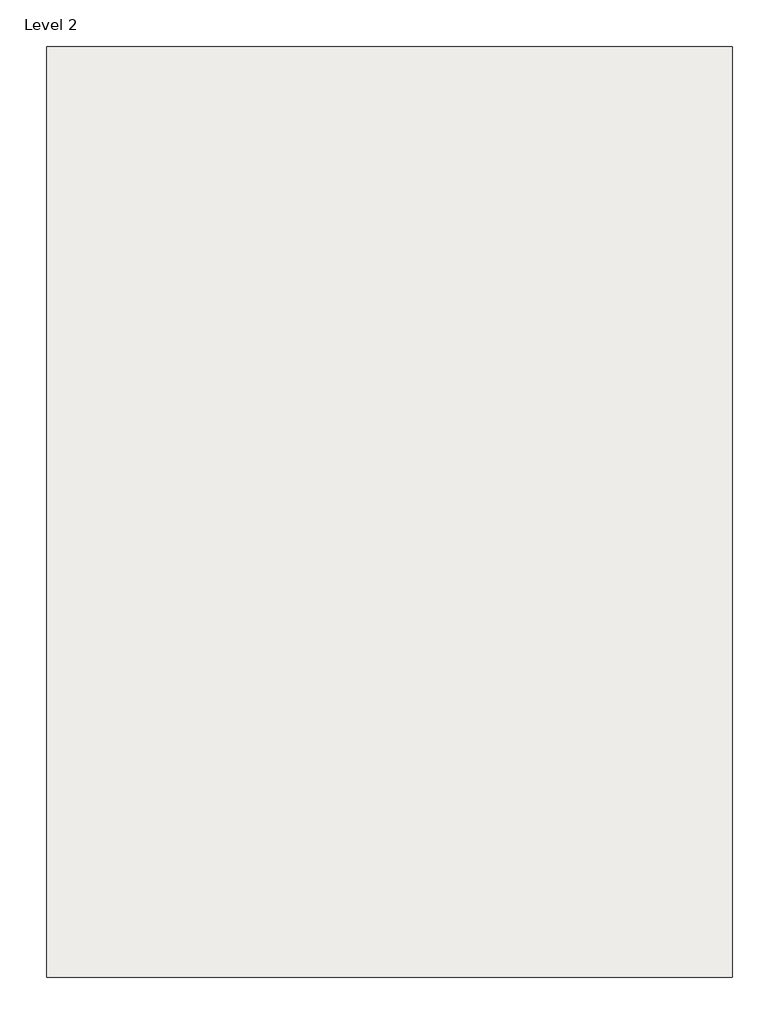
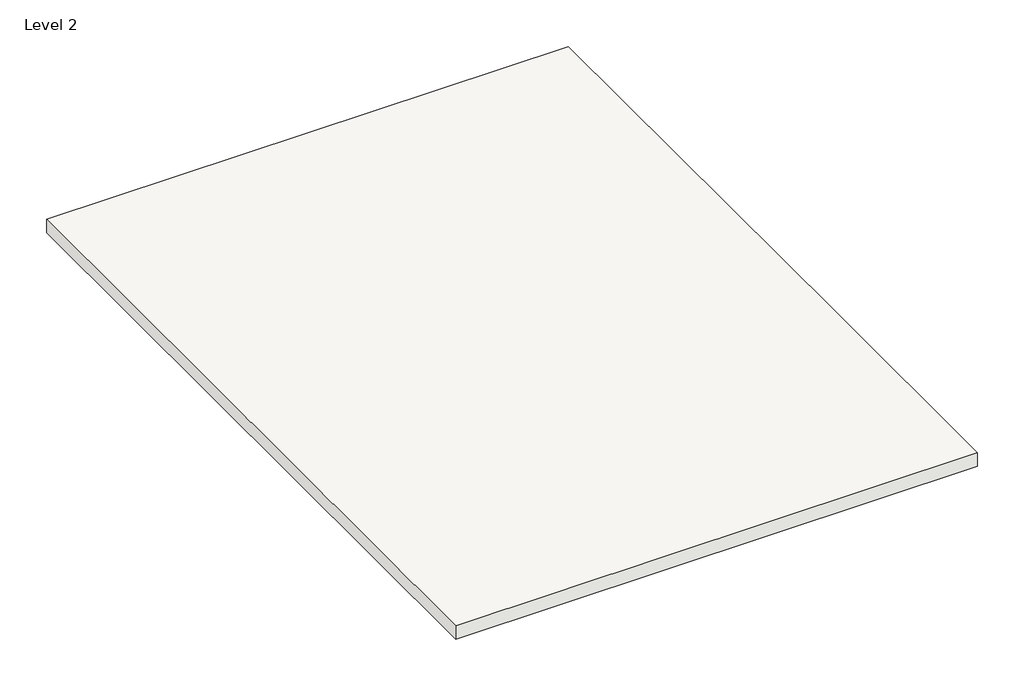
# One storey: 1 roof.
"""IFC4 building model written with IfcOpenShell, lengths in millimetres."""

from ifc_helpers import new_model, si_unit, frame, origin, place, context, project, spatial, polyline, outline, extrude, element, save

model = new_model("IFC4")

# Units and contexts
model_context = context("Model", 3, world=origin())
ifc_project = project(units=[si_unit("LENGTHUNIT", "METRE", prefix="MILLI")], contexts=[model_context])

# Site, building, storey
site = spatial("IfcSite", under=ifc_project)
building = spatial("IfcBuilding", under=site)
storey = spatial("IfcBuildingStorey", under=building, Name="Level 2", Elevation=3048.0)

# Roof
placement = place(None, origin())
element("IfcRoof", 1, ObjectType="Generic - 12\"", at=placement, inside=storey, context=model_context, shape_type="SweptSolid", body=[
    extrude(outline(polyline([(-12758.5492777, 14369.953629), (-1607.9492777, 14369.953629), (-1607.9492777, 4463.953629), (-1607.9492777, -768.446371), (-12758.5492777, -768.446371), (-12758.5492777, 14369.953629)])), frame((0.0, 0.0, 3048.0), z_axis=(0.0, 0.0, 1.0), x_axis=(1.0, 0.0, 0.0)), (0.0, 0.0, 1.0), 304.8),
])

save(model, "model.ifc")

# Revit data of these elements
# Type "Generic - 12\""
#   Assembly Code = "B1020"
#   Layers, outside or top first: 1' - 0" "Brick, Soldier Course" (function 1)
# Element 1 (IfcRoof, "Generic - 12\"")
#   built-in parameter 1001705 = 11 (stored number, unit not read)
#   built-in parameter 1001710 = 33615
#   Phase Created = New Construction
#   Materials on its faces: "Brick, Soldier Course"
# Materials
#   "Brick, Soldier Course": class "Masonry", colour RGB 170 98 104, transparency 0, Description = "Common brick soldier coursed", Cost = 0
